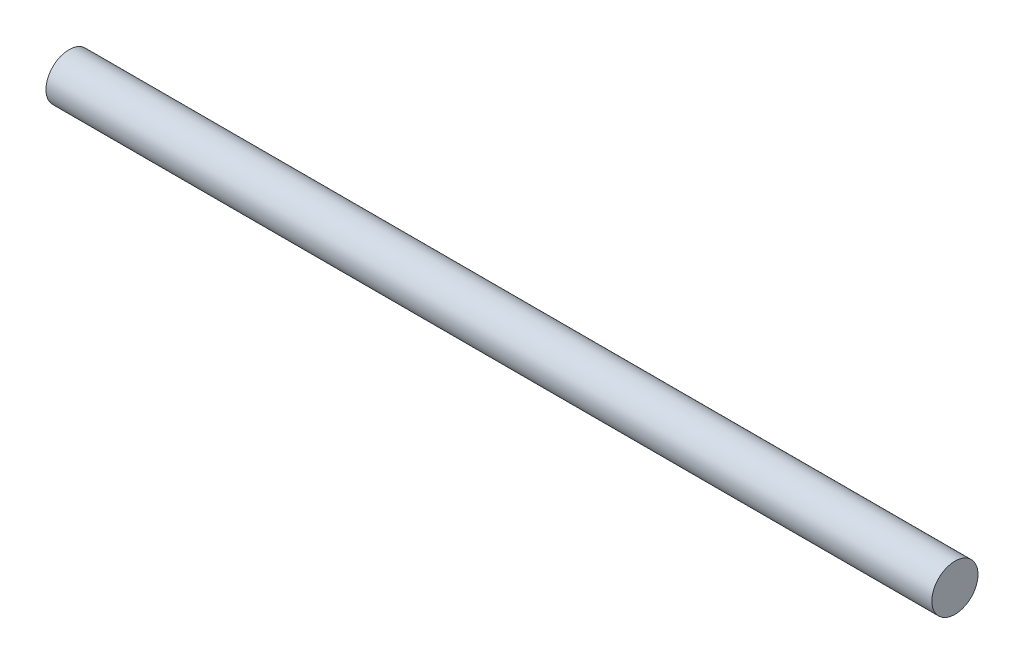
from build123d import *

# Parameters (mm, degrees)
ROD_PROFILE_5_R = 2.5
ROD_5X96_DEPTH  = 96


with BuildPart() as part:
    # Rod Profile Ø5 → Rod Ø5x96 (new body)
    with BuildSketch(Plane(origin=(0, 0, 0), x_dir=(0, 0, -1), z_dir=(1, 0, 0))):
        Circle(ROD_PROFILE_5_R)
    extrude(amount=ROD_5X96_DEPTH)


solid = part.part
